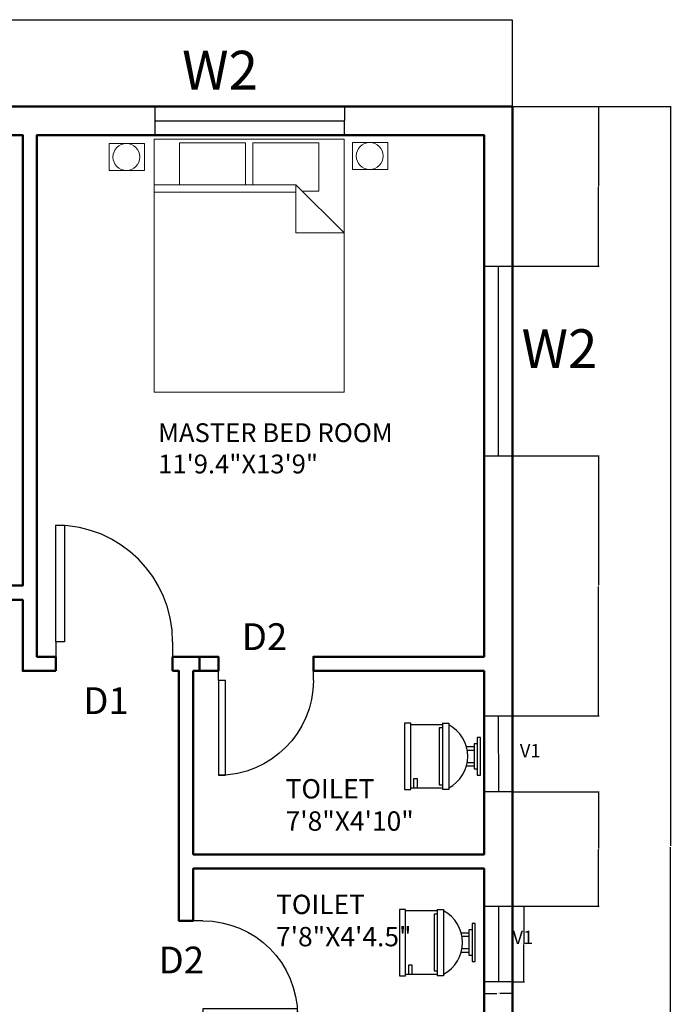
# Model space of a CAD drawing. Units: inches. Extents: x -45 to 1424, y 648 to 1662.
# Tile 7 of 8: x 1218 to 1424, y 906 to 1217. Entities that reach past the tile are written whole.
import ezdxf

# ---------------------------------------------------------------- set-up
doc = ezdxf.new("R2010")
doc.units = ezdxf.units.IN
for name, color, linetype, lineweight in [('A-ANNO-DIMS', 2, 'Continuous', 18), ('A-ANNO-TEXT', 7, 'Continuous', 18), ('A-AREA-IDEN', 7, 'Continuous', 18), ('A-FLOR-FIXT', 3, 'Continuous', 25), ('DOOR', 2, 'Continuous', 25), ('FURNITURE', 3, 'Continuous', 18), ('WALL', 4, 'Continuous', 50), ('WINDOW', 1, 'Continuous', 25)]:
    doc.layers.add(name, color=color, linetype=linetype, lineweight=lineweight)
doc.styles.get("Standard").update_dxf_attribs({"font": 'arial.ttf'})
doc.dimstyles.get("Standard").update_dxf_attribs({"dimtxt": 0.18, "dimasz": 0.18, "dimexe": 0.18, "dimexo": 0.0625, "dimgap": 0.09, "dimtad": 0, "dimtih": 1, "dimtoh": 1, "dimdec": 4, "dimzin": 0, "dimdsep": 46, "dimtxsty": 'Standard', "dimcen": 0.09, "dimadec": 0, "dimazin": 0, "dimtfac": 1, "dimtdec": 4, "dimtofl": 0, "dimtmove": 0, "dimatfit": 3, "dimfxl": 1, "dimtolj": 1, "dimtzin": 0, "dimarcsym": 0})

# ---------------------------------------------------------------- blocks, each defined once
blk = doc.blocks.new('*U3')
for p, q in [((0, 0), (0, -6)), ((24, 0), (24, -6))]:
    blk.add_line(p, q)
blk.add_lwpolyline([(0, 0), (0, 24), (1.75, 24), (1.75, 0)], close=True)
blk.add_arc((0, 0), 24, 0, 90)
blk = doc.blocks.new('*U4')
for p, q in [((-24, 0), (-24, 6)), ((0, 0), (0, 6))]:
    blk.add_line(p, q)
blk.add_lwpolyline([(0, 0), (0, -24), (-1.75, -24), (-1.75, 0)], close=True)
blk.add_arc((0, 0), 24, 180, 270)
blk = doc.blocks.new('*U5')
for p, q in [((0, 0), (0, -6)), ((24, 0), (24, -6))]:
    blk.add_line(p, q)
blk.add_lwpolyline([(0, 0), (0, 24), (1.75, 24), (1.75, 0)], close=True)
blk.add_arc((0, 0), 24, 0, 90)
blk = doc.blocks.new('Bed - Queen')
for p, q in [((0, -80.00003), (0, 0)), ((0, 0), (59.99999, 0)), ((59.99999, 0), (59.99999, -80.00003)), ((7.99999, -1.2), (28.79998, -1.2)), ((7.99999, -14.4), (7.99999, -1.2)), ((28.79998, -1.2), (28.79998, -14.4)), ((31.19999, -1.2), (51.99999, -1.2)), ((31.19999, -14.4), (31.19999, -1.2)), ((51.99999, -1.2), (51.99999, -16.4)), ((0, -14.4), (44.8, -14.4)), ((59.99999, -29.6), (44.8, -14.4)), ((44.8, -14.4), (44.8, -29.6)), ((44.8, -16.8), (0, -16.8)), ((51.99999, -16.4), (46.79936, -16.4)), ((44.8, -29.6), (59.99999, -29.6)), ((59.99999, -80.00003), (0, -80.00003))]:
    blk.add_line(p, q)
blk = doc.blocks.new('*U17')
for p, q in [((-254, 558.8), (-254, 304.8)), ((254, 304.8), (254, 558.8)), ((-254, 533.4), (-177.8, 533.4)), ((-177.8, 508), (-254, 508)), ((-177.8, 533.4), (-177.8, 508)), ((228.6, 330.2), (-228.6, 330.2)), ((-228.6, 330.2), (-228.6, 304.8)), ((228.6, 304.8), (228.6, 330.2)), ((266.7, 304.8), (-266.7, 304.8)), ((-266.7, 254), (-266.7, 304.8)), ((266.7, 254), (-266.7, 254)), ((266.7, 304.8), (266.7, 254)), ((-76.2, 111.9251), (-76.2, 50.8)), ((-50.8, 50.8), (-50.8, 105.81132)), ((50.8, 105.81132), (50.8, 50.8)), ((76.2, 50.8), (76.2, 111.9251)), ((101.6, 50.8), (-101.6, 50.8)), ((-101.6, 50.8), (-101.6, 25.4)), ((101.6, 25.4), (101.6, 50.8))]:
    blk.add_line(p, q)
for points in [[(266.7, 558.8), (266.7, 609.6), (-266.7, 609.6), (-266.7, 558.8)], [(152.4, 0), (152.4, 25.4), (-152.4, 25.4), (-152.4, 0)]]:
    blk.add_lwpolyline(points, close=True)
blk.add_arc((0, 389.46582), 287.86658, 208.0725, 331.9275)
blk = doc.blocks.new('WIN-W2-MASTER-N')
for p, q in [((0, 9), (0, 0)), ((60.08, 9), (0, 9)), ((60, 0), (60.08, 9)), ((0, 4.5), (60.04, 4.5)), ((0, 0), (60, 0))]:
    blk.add_line(p, q)
blk = doc.blocks.new('WIN-W2-MASTER-E')
for p, q in [((0, 59.99), (9, 59.99)), ((0, 0), (0, 59.99)), ((4.5, 0), (4.5, 59.99)), ((9, 0), (9, 59.99)), ((0, 0), (9, 0))]:
    blk.add_line(p, q)
blk = doc.blocks.new('VENT-V1-BATH-N')
for p, q in [((0, 24), (9, 24)), ((0, 0), (0, 24)), ((4.65, 0), (4.5, 24)), ((9, 24), (9, 0)), ((9, 0), (0, 0))]:
    blk.add_line(p, q)
blk = doc.blocks.new('VENT-V1-BATH-S')
for p, q in [((0, 24), (9, 24)), ((0, 0), (0, 24)), ((4.5, 24), (4.5, 0)), ((9, 0), (9, 24)), ((9, 0), (0, 0))]:
    blk.add_line(p, q)
blk = doc.blocks.new('FURN-BEDSIDE-UNIT')
blk.add_lwpolyline([(0, 8.55), (11.15, 8.55), (11.15, 0), (0, 0)], close=True)
blk.add_circle((5.42, 4.31), 4.24)
blk = doc.blocks.new('*D56')
at = {"layer": 'A-ANNO-DIMS', "color": 0, "lineweight": -2, "transparency": 16777216}
for p, q in [((1374.32, 936.98), (1378.03, 936.98)), ((1377.85, 936.8), (1377.85, 925.16)), ((1377.85, 913.16), (1377.85, 924.8)), ((1374.32, 912.98), (1378.03, 912.98))]:
    blk.add_line(p, q, dxfattribs=at)
at = {"layer": 'A-ANNO-DIMS', "color": 0, "transparency": 16777216}
for points in [[(1377.82, 936.8), (1377.88, 936.8), (1377.85, 936.98)], [(1377.82, 913.16), (1377.88, 913.16), (1377.85, 912.98)]]:
    blk.add_solid(points, dxfattribs=at)
at = {"layer": 'Defpoints', "color": 0, "transparency": 16777216}
for p in [(1374.25, 936.98), (1377.85, 936.98), (1374.25, 912.98)]:
    blk.add_point(p, dxfattribs=at)
at = {"layer": 'A-ANNO-DIMS', "color": 0, "transparency": 16777216, "insert": (1377.85, 924.98), "char_height": 0.18, "attachment_point": 5}
blk.add_mtext('\\A1;VENT V1 24 TYP.', dxfattribs=at)
blk = doc.blocks.new('*D57')
at = {"layer": 'A-ANNO-DIMS', "color": 0, "lineweight": -2, "transparency": 16777216}
for p, q in [((1365.25, 912.92), (1365.25, 909.2)), ((1374.25, 912.92), (1374.25, 909.2)), ((1365.43, 909.38), (1369.3, 909.38)), ((1374.07, 909.38), (1370.21, 909.38))]:
    blk.add_line(p, q, dxfattribs=at)
at = {"layer": 'A-ANNO-DIMS', "color": 0, "transparency": 16777216}
for points in [[(1365.43, 909.41), (1365.43, 909.35), (1365.25, 909.38)], [(1374.07, 909.41), (1374.07, 909.35), (1374.25, 909.38)]]:
    blk.add_solid(points, dxfattribs=at)
at = {"layer": 'Defpoints', "color": 0, "transparency": 16777216}
for p in [(1365.25, 912.98), (1374.25, 912.98), (1374.25, 909.38)]:
    blk.add_point(p, dxfattribs=at)
at = {"layer": 'A-ANNO-DIMS', "color": 0, "transparency": 16777216, "insert": (1369.75, 909.38), "char_height": 0.18, "attachment_point": 5}
blk.add_mtext('\\A1;9 TYP.', dxfattribs=at)
blk = doc.blocks.new('*D82')
at = {"layer": 'A-ANNO-DIMS', "color": 0, "lineweight": -2, "transparency": 16777216}
for p, q in [((948.85, 1189.91), (948.85, 1217.36)), ((949.03, 1217.18), (1161.16, 1217.18)), ((1374.07, 1217.18), (1161.95, 1217.18)), ((1374.25, 1189.91), (1374.25, 1217.36))]:
    blk.add_line(p, q, dxfattribs=at)
at = {"layer": 'A-ANNO-DIMS', "color": 0, "transparency": 16777216}
for points in [[(949.03, 1217.21), (949.03, 1217.15), (948.85, 1217.18)], [(1374.07, 1217.21), (1374.07, 1217.15), (1374.25, 1217.18)]]:
    blk.add_solid(points, dxfattribs=at)
at = {"layer": 'Defpoints', "color": 0, "transparency": 16777216}
for p in [(1374.25, 1217.18), (948.85, 1189.85), (1374.25, 1189.85)]:
    blk.add_point(p, dxfattribs=at)
at = {"layer": 'A-ANNO-DIMS', "color": 0, "transparency": 16777216, "insert": (1161.55, 1217.18), "char_height": 0.18, "attachment_point": 5}
blk.add_mtext('\\A1;425.4', dxfattribs=at)
blk = doc.blocks.new('*D83')
at = {"layer": 'A-ANNO-DIMS', "color": 0, "lineweight": -2, "transparency": 16777216}
for p, q in [((1374.32, 1189.85), (1424.39, 1189.85)), ((1424.21, 1189.67), (1424.21, 956.03)), ((1424.21, 722.03), (1424.21, 955.67)), ((1374.32, 721.85), (1424.39, 721.85))]:
    blk.add_line(p, q, dxfattribs=at)
at = {"layer": 'A-ANNO-DIMS', "color": 0, "transparency": 16777216}
for points in [[(1424.18, 1189.67), (1424.24, 1189.67), (1424.21, 1189.85)], [(1424.18, 722.03), (1424.24, 722.03), (1424.21, 721.85)]]:
    blk.add_solid(points, dxfattribs=at)
at = {"layer": 'Defpoints', "color": 0, "transparency": 16777216}
for p in [(1374.25, 1189.85), (1424.21, 1189.85), (1374.25, 721.85)]:
    blk.add_point(p, dxfattribs=at)
at = {"layer": 'A-ANNO-DIMS', "color": 0, "transparency": 16777216, "insert": (1424.21, 955.85), "char_height": 0.18, "attachment_point": 5}
blk.add_mtext('\\A1;468', dxfattribs=at)
blk = doc.blocks.new('*D91')
at = {"layer": 'A-ANNO-DIMS', "color": 0, "lineweight": -2, "transparency": 16777216}
for p, q in [((1374.32, 1189.85), (1401.58, 1189.85)), ((1401.4, 1189.67), (1401.4, 1164.81)), ((1401.4, 1139.59), (1401.4, 1164.45)), ((1374.32, 1139.41), (1401.58, 1139.41))]:
    blk.add_line(p, q, dxfattribs=at)
at = {"layer": 'A-ANNO-DIMS', "color": 0, "transparency": 16777216}
for points in [[(1401.37, 1189.67), (1401.43, 1189.67), (1401.4, 1189.85)], [(1401.37, 1139.59), (1401.43, 1139.59), (1401.4, 1139.41)]]:
    blk.add_solid(points, dxfattribs=at)
at = {"layer": 'Defpoints', "color": 0, "transparency": 16777216}
for p in [(1374.25, 1189.85), (1374.25, 1139.41), (1401.4, 1139.41)]:
    blk.add_point(p, dxfattribs=at)
at = {"layer": 'A-ANNO-DIMS', "color": 0, "transparency": 16777216, "insert": (1401.4, 1164.63), "char_height": 0.18, "attachment_point": 5}
blk.add_mtext('\\A1;50.44', dxfattribs=at)
blk = doc.blocks.new('*D92')
at = {"layer": 'A-ANNO-DIMS', "color": 0, "lineweight": -2, "transparency": 16777216}
for p, q in [((1374.32, 1079.42), (1401.58, 1079.42)), ((1401.4, 1079.24), (1401.4, 1038.46)), ((1401.4, 997.33), (1401.4, 1038.1)), ((1374.32, 997.15), (1401.58, 997.15))]:
    blk.add_line(p, q, dxfattribs=at)
at = {"layer": 'A-ANNO-DIMS', "color": 0, "transparency": 16777216}
for points in [[(1401.37, 1079.24), (1401.43, 1079.24), (1401.4, 1079.42)], [(1401.37, 997.33), (1401.43, 997.33), (1401.4, 997.15)]]:
    blk.add_solid(points, dxfattribs=at)
at = {"layer": 'Defpoints', "color": 0, "transparency": 16777216}
for p in [(1374.25, 1079.42), (1374.25, 997.15), (1401.4, 997.15)]:
    blk.add_point(p, dxfattribs=at)
at = {"layer": 'A-ANNO-DIMS', "color": 0, "transparency": 16777216, "insert": (1401.4, 1038.28), "char_height": 0.18, "attachment_point": 5}
blk.add_mtext('\\A1;82.27', dxfattribs=at)
blk = doc.blocks.new('*D93')
at = {"layer": 'A-ANNO-DIMS', "color": 0, "lineweight": -2, "transparency": 16777216}
for p, q in [((1374.32, 973.15), (1401.58, 973.15)), ((1401.4, 972.97), (1401.4, 955.25)), ((1401.4, 937.16), (1401.4, 954.88)), ((1374.32, 936.98), (1401.58, 936.98))]:
    blk.add_line(p, q, dxfattribs=at)
at = {"layer": 'A-ANNO-DIMS', "color": 0, "transparency": 16777216}
for points in [[(1401.37, 972.97), (1401.43, 972.97), (1401.4, 973.15)], [(1401.37, 937.16), (1401.43, 937.16), (1401.4, 936.98)]]:
    blk.add_solid(points, dxfattribs=at)
at = {"layer": 'Defpoints', "color": 0, "transparency": 16777216}
for p in [(1374.25, 973.15), (1374.25, 936.98), (1401.4, 936.98)]:
    blk.add_point(p, dxfattribs=at)
at = {"layer": 'A-ANNO-DIMS', "color": 0, "transparency": 16777216, "insert": (1401.4, 955.06), "char_height": 0.18, "attachment_point": 5}
blk.add_mtext('\\A1;36.17', dxfattribs=at)

msp = doc.modelspace()

# ---------------------------------------------------------------- linework, layer by layer
at = {"layer": 'WALL'}
for p, q in [((1229.8512, 1015.8478), (1229.8512, 1011.3478)), ((1266.755, 1015.8478), (1266.755, 1011.3478)), ((1275.2515, 1011.3478), (1275.2515, 1015.8478))]:
    msp.add_line(p, q, dxfattribs=at)
msp.add_lwpolyline([(1374.2541, 1189.8478), (1374.2541, 721.8478), (948.8541, 721.8478), (948.8541, 1189.8478)], close=True, dxfattribs=at)
for points in [[(1229.8512, 1011.3478), (1219.3541, 1011.3478), (1219.3541, 1033.8478), (1213.3544, 1033.8478), (1213.3544, 1038.3478), (1219.3541, 1038.3478), (1219.3541, 1180.8478), (1093.3541, 1180.8478), (1093.3541, 1033.8478)], [(1266.755, 1015.8478), (1281.2515, 1015.8478), (1281.2515, 1011.3478), (1273.2541, 1011.3478), (1273.2541, 953.3478), (1365.2541, 953.3478), (1365.2541, 1011.3478), (1311.2489, 1011.3478), (1311.2489, 1015.8478), (1365.2541, 1015.8478), (1365.2541, 1180.8478), (1223.8541, 1180.8478), (1223.8541, 1015.8478), (1229.8512, 1015.8478)], [(1279.2525, 896.3478), (1365.2541, 896.3478), (1365.2541, 948.8478), (1273.2541, 948.8478), (1273.2541, 932.34), (1268.7541, 932.34), (1268.7541, 1011.3478), (1266.755, 1011.3478)]]:
    msp.add_lwpolyline(points, dxfattribs=at)

# ---------------------------------------------------------------- block references
at = {"layer": 'A-FLOR-FIXT', "xscale": 0.0393700787401575, "yscale": 0.0393700787401575, "zscale": 0.0393700787401575, "rotation": 90}
for p in [(1364.0572, 984.3454), (1362.4424, 925.4521)]:
    msp.add_blockref('*U17', p, dxfattribs=at)
at = {"layer": 'DOOR'}
for name, p, xscale, yscale, zscale in [('*U3', (1229.8512, 1020.5728), 1.537499999999999, 1.537499999999999, 1.537499999999999), ('*U4', (1281.2515, 1008.3478), -1.25, 1.25, 1.25)]:
    msp.add_blockref(name, p, dxfattribs=dict(at, xscale=xscale, yscale=yscale, zscale=zscale))
at = {"layer": 'DOOR', "xscale": -1.25, "yscale": 1.25, "zscale": 1.25, "rotation": 270}
msp.add_blockref('*U5', (1276.2541, 902.3401), dxfattribs=at)
at = {"layer": 'FURNITURE'}
for name, p in [('FURN-BEDSIDE-UNIT', (1246.7057, 1169.611)), ('Bed - Queen', (1260.9547, 1179.5539)), ('FURN-BEDSIDE-UNIT', (1323.6531, 1169.9361)), ('FURN-BEDSIDE-UNIT', (1323.6531, 1169.9361))]:
    msp.add_blockref(name, p, dxfattribs=at)
at = {"layer": 'WINDOW'}
for name, p in [('WIN-W2-MASTER-N', (1261.1311, 1180.8478)), ('WIN-W2-MASTER-E', (1365.2541, 1079.4158)), ('VENT-V1-BATH-N', (1365.2541, 973.1488)), ('VENT-V1-BATH-S', (1365.2541, 912.9818))]:
    msp.add_blockref(name, p, dxfattribs=at)

# ---------------------------------------------------------------- texts
at = {"layer": 'A-ANNO-TEXT', "char_height": 12.26218, "width": 1.05025, "attachment_point": 1}
for insert in [(1269.7578, 1207.5147), (1377.0954, 1119.4304)]:
    msp.add_mtext('W2', dxfattribs=dict(at, insert=insert))
at = {"layer": 'A-ANNO-TEXT', "attachment_point": 1}
for s, width, gutter_width, insert, char_height in [('D2', 4.069942, 42.3777, (1288.625, 1026.4347), 8.47554), ('D1', 4.069942, 42.3777, (1238.5114, 1006.1927), 8.47554), ('V1', 24.172645, 21.1047, (1376.5594, 988.224), 4.22094), ('V1', 24.172645, 21.1047, (1374.2541, 929.2184), 4.22094), ('D2', 4.069942, 42.3777, (1262.3242, 924.1593), 8.47554)]:
    msp.add_mtext_dynamic_manual_height_columns(s, width=width, gutter_width=gutter_width, heights=[0], dxfattribs=dict(at, insert=insert, char_height=char_height))
at = {"layer": 'A-AREA-IDEN', "attachment_point": 1}
for s, insert, char_height in [('MASTER BED ROOM\\P11\'9.4"X13\'9"', (1262.1778, 1089.6868), 5.93871), ('TOILET\\P7\'8"X4\'10"', (1302.4804, 977.1436), 6.1222), ('TOILET\\P7\'8"X4\'4.5"', (1299.4493, 940.5839), 6.122202)]:
    msp.add_mtext(s, dxfattribs=dict(at, insert=insert, char_height=char_height))

# ---------------------------------------------------------------- dimensions: what is measured, and where the dimension line sits
at = {"layer": 'A-ANNO-DIMS'}
dim = msp.add_linear_dim(base=(1374.2541, 1217.1757), p1=(948.8541, 1189.8478), p2=(1374.2541, 1189.8478), dimstyle='Standard', override={"dimdec": 1, "dimlfac": 1, "dimrnd": 0, "dimzin": 0, "dimdsep": 46, "dimlunit": 2}, dxfattribs=at)
dim.commit()
dim.dimension.update_dxf_attribs({"geometry": '*D82', "text_midpoint": (1161.5541, 1217.1757)})
for base, p1, p2, angle, override, picture, middle in [((1424.2072, 1189.8478), (1374.2541, 721.8478), (1374.2541, 1189.8478), 90, {"dimdec": 0, "dimlfac": 1, "dimrnd": 0, "dimzin": 0, "dimdsep": 46, "dimlunit": 2}, '*D83', (1424.2072, 955.8478)), ((1401.4041, 1139.4066), (1374.2541, 1189.8478), (1374.2541, 1139.4066), 270, {"dimdec": 2, "dimlfac": 1, "dimrnd": 0, "dimzin": 0, "dimdsep": 46, "dimlunit": 2}, '*D91', (1401.4041, 1164.6272)), ((1401.4041, 997.1473), (1374.2541, 1079.4157), (1374.2541, 997.1473), 270, {"dimdec": 2, "dimlfac": 1, "dimrnd": 0, "dimzin": 0, "dimdsep": 46, "dimlunit": 2}, '*D92', (1401.4041, 1038.2815)), ((1401.4041, 936.9785), (1374.2541, 973.1491), (1374.2541, 936.9785), 270, {"dimdec": 2, "dimlfac": 1, "dimrnd": 0, "dimzin": 0, "dimdsep": 46, "dimlunit": 2}, '*D93', (1401.4041, 955.0638))]:
    dim = msp.add_linear_dim(base=base, p1=p1, p2=p2, angle=angle, dimstyle='Standard', override=override, dxfattribs=at)
    dim.commit()
    dim.dimension.update_dxf_attribs({"geometry": picture, "text_midpoint": middle})
dim = msp.add_linear_dim(base=(1377.8536, 936.9785), p1=(1374.2541, 912.9819), p2=(1374.2541, 936.9785), angle=90, text='VENT V1 <> TYP.', dimstyle='Standard', override={"dimdec": 0, "dimlfac": 1, "dimrnd": 0, "dimzin": 0, "dimdsep": 46, "dimlunit": 2}, dxfattribs=at)
dim.commit()
dim.dimension.update_dxf_attribs({"geometry": '*D56', "text_midpoint": (1377.8536, 924.9802)})
dim = msp.add_linear_dim(base=(1374.2541, 909.3825), p1=(1365.2541, 912.9819), p2=(1374.2541, 912.9819), text='<> TYP.', dimstyle='Standard', override={"dimdec": 0, "dimlfac": 1, "dimrnd": 0, "dimzin": 0, "dimdsep": 46, "dimlunit": 2}, dxfattribs=at)
dim.commit()
dim.dimension.update_dxf_attribs({"geometry": '*D57', "text_midpoint": (1369.7541, 909.3825)})

doc.saveas('drawing.dxf')
